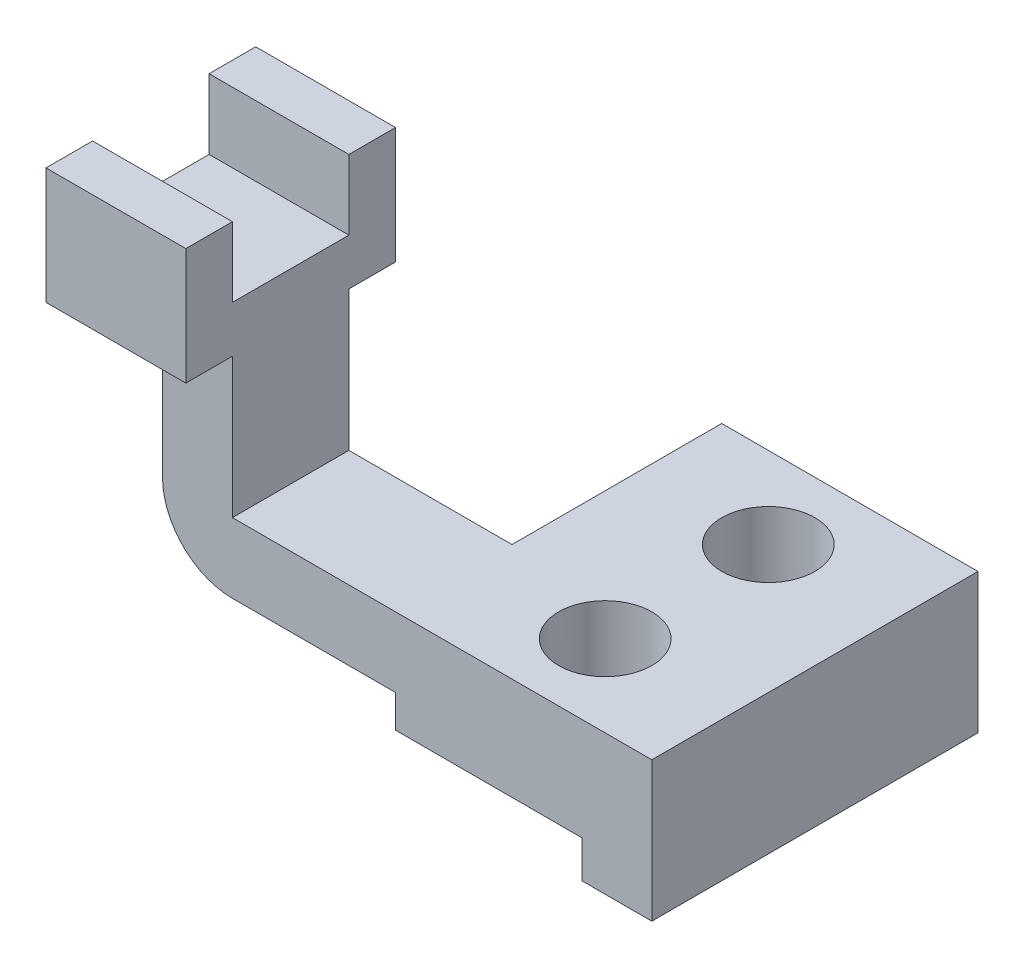
ISO-10303-21;
HEADER;
FILE_DESCRIPTION(('STEP AP214'),'2;1');
FILE_NAME('part.step','',(''),(''),'','','');
FILE_SCHEMA(('AUTOMOTIVE_DESIGN { 1 0 10303 214 1 1 1 1 }'));
ENDSEC;
DATA;
#1=APPLICATION_CONTEXT('core data for automotive mechanical design processes');
#2=APPLICATION_PROTOCOL_DEFINITION('international standard','automotive_design',2000,#1);
#3=PRODUCT_CONTEXT('',#1,'mechanical');
#4=PRODUCT('Part','Part','',(#3));
#5=PRODUCT_RELATED_PRODUCT_CATEGORY('part','',(#4));
#6=PRODUCT_DEFINITION_FORMATION('','',#4);
#7=PRODUCT_DEFINITION_CONTEXT('part definition',#1,'design');
#8=PRODUCT_DEFINITION('design','',#6,#7);
#9=PRODUCT_DEFINITION_SHAPE('','',#8);
#10=(LENGTH_UNIT() NAMED_UNIT(*) SI_UNIT(.MILLI.,.METRE.));
#11=(NAMED_UNIT(*) PLANE_ANGLE_UNIT() SI_UNIT($,.RADIAN.));
#12=(NAMED_UNIT(*) SI_UNIT($,.STERADIAN.) SOLID_ANGLE_UNIT());
#13=UNCERTAINTY_MEASURE_WITH_UNIT(LENGTH_MEASURE(1.E-05),#10,'distance_accuracy_value','');
#14=(GEOMETRIC_REPRESENTATION_CONTEXT(3) GLOBAL_UNCERTAINTY_ASSIGNED_CONTEXT((#13)) GLOBAL_UNIT_ASSIGNED_CONTEXT((#10,
#11,#12)) REPRESENTATION_CONTEXT('',''));
#15=CARTESIAN_POINT('',(0.,0.,0.));
#16=DIRECTION('',(0.,0.,1.));
#17=DIRECTION('',(1.,0.,0.));
#18=AXIS2_PLACEMENT_3D('',#15,#16,#17);
#19=CARTESIAN_POINT('',(-27500.,0.,35000.));
#20=DIRECTION('',(-1.,0.,0.));
#21=DIRECTION('',(0.,0.,1.));
#22=AXIS2_PLACEMENT_3D('',#19,#20,#21);
#23=PLANE('',#22);
#24=DIRECTION('',(0.,1.,0.));
#25=VECTOR('',#24,1.);
#26=CARTESIAN_POINT('',(-27500.,0.,35000.));
#27=LINE('',#26,#25);
#28=CARTESIAN_POINT('',(-27500.,-7000.,35000.));
#29=VERTEX_POINT('',#28);
#30=CARTESIAN_POINT('',(-27500.,-1.77635683940025E-12,35000.));
#31=VERTEX_POINT('',#30);
#32=EDGE_CURVE('E316',#29,#31,#27,.T.);
#33=ORIENTED_EDGE('',*,*,#32,.T.);
#34=DIRECTION('',(0.,0.,-1.));
#35=VECTOR('',#34,1.);
#36=CARTESIAN_POINT('',(-27500.,-1.77635683940025E-12,35000.));
#37=LINE('',#36,#35);
#38=CARTESIAN_POINT('',(-27500.,-1.77635683940025E-12,10000.));
#39=VERTEX_POINT('',#38);
#40=EDGE_CURVE('E282',#31,#39,#37,.T.);
#41=ORIENTED_EDGE('',*,*,#40,.T.);
#42=DIRECTION('',(0.,1.,0.));
#43=VECTOR('',#42,1.);
#44=CARTESIAN_POINT('',(-27500.,-1.77635683940025E-12,10000.));
#45=LINE('',#44,#43);
#46=CARTESIAN_POINT('',(-27500.,15000.,10000.));
#47=VERTEX_POINT('',#46);
#48=EDGE_CURVE('E292',#39,#47,#45,.T.);
#49=ORIENTED_EDGE('',*,*,#48,.T.);
#50=DIRECTION('',(0.,0.,-1.));
#51=VECTOR('',#50,1.);
#52=CARTESIAN_POINT('',(-27500.,15000.,35000.));
#53=LINE('',#52,#51);
#54=CARTESIAN_POINT('',(-27500.,15000.,-35000.));
#55=VERTEX_POINT('',#54);
#56=EDGE_CURVE('E340',#47,#55,#53,.T.);
#57=ORIENTED_EDGE('',*,*,#56,.T.);
#58=DIRECTION('',(0.,1.,0.));
#59=VECTOR('',#58,1.);
#60=CARTESIAN_POINT('',(-27500.,0.,-35000.));
#61=LINE('',#60,#59);
#62=CARTESIAN_POINT('',(-27500.,-7000.,-35000.));
#63=VERTEX_POINT('',#62);
#64=EDGE_CURVE('E304',#63,#55,#61,.T.);
#65=ORIENTED_EDGE('',*,*,#64,.F.);
#66=DIRECTION('',(0.,0.,-1.));
#67=VECTOR('',#66,1.);
#68=CARTESIAN_POINT('',(-27500.,-7000.,35000.));
#69=LINE('',#68,#67);
#70=EDGE_CURVE('E317',#29,#63,#69,.T.);
#71=ORIENTED_EDGE('',*,*,#70,.F.);
#72=EDGE_LOOP('',(#33,#41,#49,#57,#65,#71));
#73=FACE_BOUND('',#72,.T.);
#74=ADVANCED_FACE('F47',(#73),#23,.T.);
#75=CARTESIAN_POINT('',(9.32587340685132E-13,-7000.,35000.));
#76=DIRECTION('',(0.,-1.,0.));
#77=DIRECTION('',(1.,0.,0.));
#78=AXIS2_PLACEMENT_3D('',#75,#76,#77);
#79=PLANE('',#78);
#80=CARTESIAN_POINT('',(0.,-7000.,-17500.));
#81=DIRECTION('',(0.,-1.,0.));
#82=DIRECTION('',(1.,0.,0.));
#83=AXIS2_PLACEMENT_3D('',#80,#81,#82);
#84=CIRCLE('',#83,10000.);
#85=CARTESIAN_POINT('',(10000.,-7000.,-17500.));
#86=VERTEX_POINT('',#85);
#87=EDGE_CURVE('E217',#86,#86,#84,.T.);
#88=ORIENTED_EDGE('',*,*,#87,.F.);
#89=EDGE_LOOP('',(#88));
#90=FACE_BOUND('',#89,.T.);
#91=CARTESIAN_POINT('',(2.14313189850787E-12,-7000.,17500.));
#92=DIRECTION('',(0.,-1.,0.));
#93=DIRECTION('',(1.,0.,0.));
#94=AXIS2_PLACEMENT_3D('',#91,#92,#93);
#95=CIRCLE('',#94,10000.);
#96=CARTESIAN_POINT('',(10000.,-7000.,17500.));
#97=VERTEX_POINT('',#96);
#98=EDGE_CURVE('E743',#97,#97,#95,.T.);
#99=ORIENTED_EDGE('',*,*,#98,.F.);
#100=EDGE_LOOP('',(#99));
#101=FACE_BOUND('',#100,.T.);
#102=DIRECTION('',(-1.,0.,0.));
#103=VECTOR('',#102,1.);
#104=CARTESIAN_POINT('',(9.32587340685132E-13,-7000.,-35000.));
#105=LINE('',#104,#103);
#106=CARTESIAN_POINT('',(12500.,-7000.,-35000.));
#107=VERTEX_POINT('',#106);
#108=EDGE_CURVE('E293',#107,#63,#105,.T.);
#109=ORIENTED_EDGE('',*,*,#108,.F.);
#110=DIRECTION('',(0.,0.,-1.));
#111=VECTOR('',#110,1.);
#112=CARTESIAN_POINT('',(12500.,-7000.,35000.));
#113=LINE('',#112,#111);
#114=CARTESIAN_POINT('',(12500.,-7000.,35000.));
#115=VERTEX_POINT('',#114);
#116=EDGE_CURVE('E344',#115,#107,#113,.T.);
#117=ORIENTED_EDGE('',*,*,#116,.F.);
#118=DIRECTION('',(-1.,0.,0.));
#119=VECTOR('',#118,1.);
#120=CARTESIAN_POINT('',(9.32587340685132E-13,-7000.,35000.));
#121=LINE('',#120,#119);
#122=EDGE_CURVE('E301',#115,#29,#121,.T.);
#123=ORIENTED_EDGE('',*,*,#122,.T.);
#124=ORIENTED_EDGE('',*,*,#70,.T.);
#125=EDGE_LOOP('',(#109,#117,#123,#124));
#126=FACE_BOUND('',#125,.T.);
#127=ADVANCED_FACE('F380',(#90,#101,#126),#79,.T.);
#128=CARTESIAN_POINT('',(12500.,0.,35000.));
#129=DIRECTION('',(-1.,0.,0.));
#130=DIRECTION('',(0.,0.,1.));
#131=AXIS2_PLACEMENT_3D('',#128,#129,#130);
#132=PLANE('',#131);
#133=DIRECTION('',(0.,1.,0.));
#134=VECTOR('',#133,1.);
#135=CARTESIAN_POINT('',(12500.,0.,-35000.));
#136=LINE('',#135,#134);
#137=CARTESIAN_POINT('',(12500.,-15000.,-35000.));
#138=VERTEX_POINT('',#137);
#139=EDGE_CURVE('E325',#138,#107,#136,.T.);
#140=ORIENTED_EDGE('',*,*,#139,.F.);
#141=DIRECTION('',(0.,0.,-1.));
#142=VECTOR('',#141,1.);
#143=CARTESIAN_POINT('',(12500.,-15000.,35000.));
#144=LINE('',#143,#142);
#145=CARTESIAN_POINT('',(12500.,-15000.,35000.));
#146=VERTEX_POINT('',#145);
#147=EDGE_CURVE('E343',#146,#138,#144,.T.);
#148=ORIENTED_EDGE('',*,*,#147,.F.);
#149=DIRECTION('',(0.,1.,0.));
#150=VECTOR('',#149,1.);
#151=CARTESIAN_POINT('',(12500.,0.,35000.));
#152=LINE('',#151,#150);
#153=EDGE_CURVE('E302',#146,#115,#152,.T.);
#154=ORIENTED_EDGE('',*,*,#153,.T.);
#155=ORIENTED_EDGE('',*,*,#116,.T.);
#156=EDGE_LOOP('',(#140,#148,#154,#155));
#157=FACE_BOUND('',#156,.T.);
#158=ADVANCED_FACE('F382',(#157),#132,.T.);
#159=CARTESIAN_POINT('',(0.,-15000.,35000.));
#160=DIRECTION('',(0.,-1.,0.));
#161=DIRECTION('',(0.,0.,-1.));
#162=AXIS2_PLACEMENT_3D('',#159,#160,#161);
#163=PLANE('',#162);
#164=DIRECTION('',(-1.,0.,0.));
#165=VECTOR('',#164,1.);
#166=CARTESIAN_POINT('',(0.,-15000.,-35000.));
#167=LINE('',#166,#165);
#168=CARTESIAN_POINT('',(27500.,-15000.,-35000.));
#169=VERTEX_POINT('',#168);
#170=EDGE_CURVE('E324',#169,#138,#167,.T.);
#171=ORIENTED_EDGE('',*,*,#170,.F.);
#172=DIRECTION('',(0.,0.,-1.));
#173=VECTOR('',#172,1.);
#174=CARTESIAN_POINT('',(27500.,-15000.,35000.));
#175=LINE('',#174,#173);
#176=CARTESIAN_POINT('',(27500.,-15000.,35000.));
#177=VERTEX_POINT('',#176);
#178=EDGE_CURVE('E341',#177,#169,#175,.T.);
#179=ORIENTED_EDGE('',*,*,#178,.F.);
#180=DIRECTION('',(-1.,0.,0.));
#181=VECTOR('',#180,1.);
#182=CARTESIAN_POINT('',(0.,-15000.,35000.));
#183=LINE('',#182,#181);
#184=EDGE_CURVE('E306',#177,#146,#183,.T.);
#185=ORIENTED_EDGE('',*,*,#184,.T.);
#186=ORIENTED_EDGE('',*,*,#147,.T.);
#187=EDGE_LOOP('',(#171,#179,#185,#186));
#188=FACE_BOUND('',#187,.T.);
#189=ADVANCED_FACE('F396',(#188),#163,.T.);
#190=CARTESIAN_POINT('',(27500.,6.51330841113425E-12,35000.));
#191=DIRECTION('',(1.,0.,0.));
#192=DIRECTION('',(0.,1.,0.));
#193=AXIS2_PLACEMENT_3D('',#190,#191,#192);
#194=PLANE('',#193);
#195=DIRECTION('',(0.,-1.,0.));
#196=VECTOR('',#195,1.);
#197=CARTESIAN_POINT('',(27500.,6.51330841113425E-12,-35000.));
#198=LINE('',#197,#196);
#199=CARTESIAN_POINT('',(27500.,15000.,-35000.));
#200=VERTEX_POINT('',#199);
#201=EDGE_CURVE('E327',#200,#169,#198,.T.);
#202=ORIENTED_EDGE('',*,*,#201,.F.);
#203=DIRECTION('',(0.,0.,-1.));
#204=VECTOR('',#203,1.);
#205=CARTESIAN_POINT('',(27500.,15000.,35000.));
#206=LINE('',#205,#204);
#207=CARTESIAN_POINT('',(27500.,15000.,35000.));
#208=VERTEX_POINT('',#207);
#209=EDGE_CURVE('E337',#208,#200,#206,.T.);
#210=ORIENTED_EDGE('',*,*,#209,.F.);
#211=DIRECTION('',(0.,-1.,0.));
#212=VECTOR('',#211,1.);
#213=CARTESIAN_POINT('',(27500.,6.51330841113425E-12,35000.));
#214=LINE('',#213,#212);
#215=EDGE_CURVE('E313',#208,#177,#214,.T.);
#216=ORIENTED_EDGE('',*,*,#215,.T.);
#217=ORIENTED_EDGE('',*,*,#178,.T.);
#218=EDGE_LOOP('',(#202,#210,#216,#217));
#219=FACE_BOUND('',#218,.T.);
#220=ADVANCED_FACE('F395',(#219),#194,.T.);
#221=CARTESIAN_POINT('',(0.,15000.,35000.));
#222=DIRECTION('',(0.,1.,0.));
#223=DIRECTION('',(0.,0.,1.));
#224=AXIS2_PLACEMENT_3D('',#221,#222,#223);
#225=PLANE('',#224);
#226=CARTESIAN_POINT('',(0.,15000.,-17500.));
#227=DIRECTION('',(0.,1.,0.));
#228=DIRECTION('',(0.,0.,1.));
#229=AXIS2_PLACEMENT_3D('',#226,#227,#228);
#230=CIRCLE('',#229,10000.);
#231=CARTESIAN_POINT('',(0.,15000.,-7500.));
#232=VERTEX_POINT('',#231);
#233=EDGE_CURVE('E745',#232,#232,#230,.T.);
#234=ORIENTED_EDGE('',*,*,#233,.F.);
#235=EDGE_LOOP('',(#234));
#236=FACE_BOUND('',#235,.T.);
#237=CARTESIAN_POINT('',(2.14313189850787E-12,15000.,17500.));
#238=DIRECTION('',(0.,1.,0.));
#239=DIRECTION('',(0.,0.,1.));
#240=AXIS2_PLACEMENT_3D('',#237,#238,#239);
#241=CIRCLE('',#240,10000.);
#242=CARTESIAN_POINT('',(2.14313189850787E-12,15000.,27500.));
#243=VERTEX_POINT('',#242);
#244=EDGE_CURVE('E742',#243,#243,#241,.T.);
#245=ORIENTED_EDGE('',*,*,#244,.F.);
#246=EDGE_LOOP('',(#245));
#247=FACE_BOUND('',#246,.T.);
#248=DIRECTION('',(0.,0.,-1.));
#249=VECTOR('',#248,1.);
#250=CARTESIAN_POINT('',(-62500.,15000.,35000.));
#251=LINE('',#250,#249);
#252=CARTESIAN_POINT('',(-62500.,15000.,35000.));
#253=VERTEX_POINT('',#252);
#254=CARTESIAN_POINT('',(-62500.,15000.,10000.));
#255=VERTEX_POINT('',#254);
#256=EDGE_CURVE('E255',#253,#255,#251,.T.);
#257=ORIENTED_EDGE('',*,*,#256,.F.);
#258=DIRECTION('',(1.,0.,0.));
#259=VECTOR('',#258,1.);
#260=CARTESIAN_POINT('',(0.,15000.,35000.));
#261=LINE('',#260,#259);
#262=EDGE_CURVE('E314',#253,#208,#261,.T.);
#263=ORIENTED_EDGE('',*,*,#262,.T.);
#264=ORIENTED_EDGE('',*,*,#209,.T.);
#265=DIRECTION('',(1.,0.,0.));
#266=VECTOR('',#265,1.);
#267=CARTESIAN_POINT('',(0.,15000.,-35000.));
#268=LINE('',#267,#266);
#269=EDGE_CURVE('E332',#55,#200,#268,.T.);
#270=ORIENTED_EDGE('',*,*,#269,.F.);
#271=ORIENTED_EDGE('',*,*,#56,.F.);
#272=DIRECTION('',(-1.,0.,0.));
#273=VECTOR('',#272,1.);
#274=CARTESIAN_POINT('',(-27500.,15000.,10000.));
#275=LINE('',#274,#273);
#276=EDGE_CURVE('E281',#47,#255,#275,.T.);
#277=ORIENTED_EDGE('',*,*,#276,.T.);
#278=EDGE_LOOP('',(#257,#263,#264,#270,#271,#277));
#279=FACE_BOUND('',#278,.T.);
#280=ADVANCED_FACE('F386',(#236,#247,#279),#225,.T.);
#281=CARTESIAN_POINT('',(0.,0.,35000.));
#282=DIRECTION('',(0.,0.,1.));
#283=DIRECTION('',(1.,0.,0.));
#284=AXIS2_PLACEMENT_3D('',#281,#282,#283);
#285=PLANE('',#284);
#286=DIRECTION('',(0.,1.,0.));
#287=VECTOR('',#286,1.);
#288=CARTESIAN_POINT('',(-77500.,-1.77635683940025E-12,35000.));
#289=LINE('',#288,#287);
#290=CARTESIAN_POINT('',(-77500.,15000.,35000.));
#291=VERTEX_POINT('',#290);
#292=CARTESIAN_POINT('',(-77500.,45000.,35000.));
#293=VERTEX_POINT('',#292);
#294=EDGE_CURVE('E291',#291,#293,#289,.T.);
#295=ORIENTED_EDGE('',*,*,#294,.F.);
#296=CARTESIAN_POINT('',(-62500.,15000.,35000.));
#297=DIRECTION('',(0.,0.,1.));
#298=DIRECTION('',(1.,0.,0.));
#299=AXIS2_PLACEMENT_3D('',#296,#297,#298);
#300=CIRCLE('',#299,15000.);
#301=CARTESIAN_POINT('',(-62500.,-1.77635683940025E-12,35000.));
#302=VERTEX_POINT('',#301);
#303=EDGE_CURVE('E72',#291,#302,#300,.T.);
#304=ORIENTED_EDGE('',*,*,#303,.T.);
#305=DIRECTION('',(1.,0.,0.));
#306=VECTOR('',#305,1.);
#307=CARTESIAN_POINT('',(-27500.,-1.77635683940025E-12,35000.));
#308=LINE('',#307,#306);
#309=EDGE_CURVE('E287',#302,#31,#308,.T.);
#310=ORIENTED_EDGE('',*,*,#309,.T.);
#311=ORIENTED_EDGE('',*,*,#32,.F.);
#312=ORIENTED_EDGE('',*,*,#122,.F.);
#313=ORIENTED_EDGE('',*,*,#153,.F.);
#314=ORIENTED_EDGE('',*,*,#184,.F.);
#315=ORIENTED_EDGE('',*,*,#215,.F.);
#316=ORIENTED_EDGE('',*,*,#262,.F.);
#317=DIRECTION('',(0.,-1.,0.));
#318=VECTOR('',#317,1.);
#319=CARTESIAN_POINT('',(-62500.,45000.,35000.));
#320=LINE('',#319,#318);
#321=CARTESIAN_POINT('',(-62500.,45000.,35000.));
#322=VERTEX_POINT('',#321);
#323=EDGE_CURVE('E278',#322,#253,#320,.T.);
#324=ORIENTED_EDGE('',*,*,#323,.F.);
#325=DIRECTION('',(1.,0.,0.));
#326=VECTOR('',#325,1.);
#327=CARTESIAN_POINT('',(-77500.,45000.,35000.));
#328=LINE('',#327,#326);
#329=EDGE_CURVE('E267',#293,#322,#328,.T.);
#330=ORIENTED_EDGE('',*,*,#329,.F.);
#331=EDGE_LOOP('',(#295,#304,#310,#311,#312,#313,#314,#315,#316,#324,#330));
#332=FACE_BOUND('',#331,.T.);
#333=ADVANCED_FACE('F360',(#332),#285,.T.);
#334=CARTESIAN_POINT('',(0.,0.,-35000.));
#335=DIRECTION('',(0.,0.,1.));
#336=DIRECTION('',(1.,0.,0.));
#337=AXIS2_PLACEMENT_3D('',#334,#335,#336);
#338=PLANE('',#337);
#339=ORIENTED_EDGE('',*,*,#108,.T.);
#340=ORIENTED_EDGE('',*,*,#64,.T.);
#341=ORIENTED_EDGE('',*,*,#269,.T.);
#342=ORIENTED_EDGE('',*,*,#201,.T.);
#343=ORIENTED_EDGE('',*,*,#170,.T.);
#344=ORIENTED_EDGE('',*,*,#139,.T.);
#345=EDGE_LOOP('',(#339,#340,#341,#342,#343,#344));
#346=FACE_BOUND('',#345,.T.);
#347=ADVANCED_FACE('F390',(#346),#338,.F.);
#348=CARTESIAN_POINT('',(-77500.,-1.77635683940025E-12,35000.));
#349=DIRECTION('',(-1.,0.,0.));
#350=DIRECTION('',(0.,0.,1.));
#351=AXIS2_PLACEMENT_3D('',#348,#349,#350);
#352=PLANE('',#351);
#353=DIRECTION('',(0.,1.,0.));
#354=VECTOR('',#353,1.);
#355=CARTESIAN_POINT('',(-77500.,-1.77635683940025E-12,10000.));
#356=LINE('',#355,#354);
#357=CARTESIAN_POINT('',(-77500.,15000.,10000.));
#358=VERTEX_POINT('',#357);
#359=CARTESIAN_POINT('',(-77500.,45000.,10000.));
#360=VERTEX_POINT('',#359);
#361=EDGE_CURVE('E298',#358,#360,#356,.T.);
#362=ORIENTED_EDGE('',*,*,#361,.F.);
#363=DIRECTION('',(0.,0.,1.));
#364=VECTOR('',#363,1.);
#365=CARTESIAN_POINT('',(-77500.,15000.,35000.));
#366=LINE('',#365,#364);
#367=EDGE_CURVE('E350',#358,#291,#366,.T.);
#368=ORIENTED_EDGE('',*,*,#367,.T.);
#369=ORIENTED_EDGE('',*,*,#294,.T.);
#370=DIRECTION('',(0.,0.,1.));
#371=VECTOR('',#370,1.);
#372=CARTESIAN_POINT('',(-77500.,45000.,35000.));
#373=LINE('',#372,#371);
#374=EDGE_CURVE('E266',#360,#293,#373,.T.);
#375=ORIENTED_EDGE('',*,*,#374,.F.);
#376=EDGE_LOOP('',(#362,#368,#369,#375));
#377=FACE_BOUND('',#376,.T.);
#378=ADVANCED_FACE('F351',(#377),#352,.T.);
#379=CARTESIAN_POINT('',(-27500.,-1.77635683940025E-12,10000.));
#380=DIRECTION('',(0.,0.,-1.));
#381=DIRECTION('',(-1.,0.,0.));
#382=AXIS2_PLACEMENT_3D('',#379,#380,#381);
#383=PLANE('',#382);
#384=DIRECTION('',(-1.,0.,0.));
#385=VECTOR('',#384,1.);
#386=CARTESIAN_POINT('',(-27500.,-1.77635683940025E-12,10000.));
#387=LINE('',#386,#385);
#388=CARTESIAN_POINT('',(-62500.,-1.77635683940025E-12,10000.));
#389=VERTEX_POINT('',#388);
#390=EDGE_CURVE('E290',#39,#389,#387,.T.);
#391=ORIENTED_EDGE('',*,*,#390,.T.);
#392=CARTESIAN_POINT('',(-62500.,15000.,10000.));
#393=DIRECTION('',(0.,0.,-1.));
#394=DIRECTION('',(-1.,0.,0.));
#395=AXIS2_PLACEMENT_3D('',#392,#393,#394);
#396=CIRCLE('',#395,15000.);
#397=EDGE_CURVE('E11',#389,#358,#396,.T.);
#398=ORIENTED_EDGE('',*,*,#397,.T.);
#399=ORIENTED_EDGE('',*,*,#361,.T.);
#400=DIRECTION('',(-1.,0.,0.));
#401=VECTOR('',#400,1.);
#402=CARTESIAN_POINT('',(-77500.,45000.,10000.));
#403=LINE('',#402,#401);
#404=CARTESIAN_POINT('',(-62500.,45000.,10000.));
#405=VERTEX_POINT('',#404);
#406=EDGE_CURVE('E275',#405,#360,#403,.T.);
#407=ORIENTED_EDGE('',*,*,#406,.F.);
#408=DIRECTION('',(0.,-1.,0.));
#409=VECTOR('',#408,1.);
#410=CARTESIAN_POINT('',(-62500.,45000.,10000.));
#411=LINE('',#410,#409);
#412=EDGE_CURVE('E274',#405,#255,#411,.T.);
#413=ORIENTED_EDGE('',*,*,#412,.T.);
#414=ORIENTED_EDGE('',*,*,#276,.F.);
#415=ORIENTED_EDGE('',*,*,#48,.F.);
#416=EDGE_LOOP('',(#391,#398,#399,#407,#413,#414,#415));
#417=FACE_BOUND('',#416,.T.);
#418=ADVANCED_FACE('F364',(#417),#383,.T.);
#419=CARTESIAN_POINT('',(0.,-1.77635683940025E-12,0.));
#420=DIRECTION('',(0.,1.,0.));
#421=DIRECTION('',(0.,0.,1.));
#422=AXIS2_PLACEMENT_3D('',#419,#420,#421);
#423=PLANE('',#422);
#424=ORIENTED_EDGE('',*,*,#309,.F.);
#425=DIRECTION('',(0.,0.,1.));
#426=VECTOR('',#425,1.);
#427=CARTESIAN_POINT('',(-62500.,-1.77635683940025E-12,10000.));
#428=LINE('',#427,#426);
#429=EDGE_CURVE('E60',#302,#389,#428,.F.);
#430=ORIENTED_EDGE('',*,*,#429,.T.);
#431=ORIENTED_EDGE('',*,*,#390,.F.);
#432=ORIENTED_EDGE('',*,*,#40,.F.);
#433=EDGE_LOOP('',(#424,#430,#431,#432));
#434=FACE_BOUND('',#433,.T.);
#435=ADVANCED_FACE('F373',(#434),#423,.F.);
#436=CARTESIAN_POINT('',(-62500.,45000.,35000.));
#437=DIRECTION('',(-1.,0.,0.));
#438=DIRECTION('',(0.,0.,1.));
#439=AXIS2_PLACEMENT_3D('',#436,#437,#438);
#440=PLANE('',#439);
#441=ORIENTED_EDGE('',*,*,#256,.T.);
#442=ORIENTED_EDGE('',*,*,#412,.F.);
#443=DIRECTION('',(0.,0.,-1.));
#444=VECTOR('',#443,1.);
#445=CARTESIAN_POINT('',(-62500.,45000.,1.4210854715202E-11));
#446=LINE('',#445,#444);
#447=CARTESIAN_POINT('',(-62500.,45000.,1.4210854715202E-11));
#448=VERTEX_POINT('',#447);
#449=EDGE_CURVE('E214',#405,#448,#446,.T.);
#450=ORIENTED_EDGE('',*,*,#449,.T.);
#451=DIRECTION('',(0.,1.,0.));
#452=VECTOR('',#451,1.);
#453=CARTESIAN_POINT('',(-62500.,45000.,1.4210854715202E-11));
#454=LINE('',#453,#452);
#455=CARTESIAN_POINT('',(-62500.,70000.,1.4210854715202E-11));
#456=VERTEX_POINT('',#455);
#457=EDGE_CURVE('E234',#448,#456,#454,.T.);
#458=ORIENTED_EDGE('',*,*,#457,.T.);
#459=DIRECTION('',(0.,0.,1.));
#460=VECTOR('',#459,1.);
#461=CARTESIAN_POINT('',(-62500.,70000.,1.4210854715202E-11));
#462=LINE('',#461,#460);
#463=CARTESIAN_POINT('',(-62500.,70000.,10000.));
#464=VERTEX_POINT('',#463);
#465=EDGE_CURVE('E189',#456,#464,#462,.T.);
#466=ORIENTED_EDGE('',*,*,#465,.T.);
#467=DIRECTION('',(0.,-1.,0.));
#468=VECTOR('',#467,1.);
#469=CARTESIAN_POINT('',(-62500.,70000.,10000.));
#470=LINE('',#469,#468);
#471=CARTESIAN_POINT('',(-62500.,55000.,10000.));
#472=VERTEX_POINT('',#471);
#473=EDGE_CURVE('E236',#464,#472,#470,.T.);
#474=ORIENTED_EDGE('',*,*,#473,.T.);
#475=DIRECTION('',(0.,0.,1.));
#476=VECTOR('',#475,1.);
#477=CARTESIAN_POINT('',(-62500.,55000.,10000.));
#478=LINE('',#477,#476);
#479=CARTESIAN_POINT('',(-62500.,55000.,35000.));
#480=VERTEX_POINT('',#479);
#481=EDGE_CURVE('E243',#472,#480,#478,.T.);
#482=ORIENTED_EDGE('',*,*,#481,.T.);
#483=DIRECTION('',(0.,1.,0.));
#484=VECTOR('',#483,1.);
#485=CARTESIAN_POINT('',(-62500.,55000.,35000.));
#486=LINE('',#485,#484);
#487=CARTESIAN_POINT('',(-62500.,70000.,35000.));
#488=VERTEX_POINT('',#487);
#489=EDGE_CURVE('E242',#480,#488,#486,.T.);
#490=ORIENTED_EDGE('',*,*,#489,.T.);
#491=DIRECTION('',(0.,0.,1.));
#492=VECTOR('',#491,1.);
#493=CARTESIAN_POINT('',(-62500.,70000.,35000.));
#494=LINE('',#493,#492);
#495=CARTESIAN_POINT('',(-62500.,70000.,45000.));
#496=VERTEX_POINT('',#495);
#497=EDGE_CURVE('E250',#488,#496,#494,.T.);
#498=ORIENTED_EDGE('',*,*,#497,.T.);
#499=DIRECTION('',(0.,-1.,0.));
#500=VECTOR('',#499,1.);
#501=CARTESIAN_POINT('',(-62500.,45000.,45000.));
#502=LINE('',#501,#500);
#503=CARTESIAN_POINT('',(-62500.,45000.,45000.));
#504=VERTEX_POINT('',#503);
#505=EDGE_CURVE('E249',#496,#504,#502,.T.);
#506=ORIENTED_EDGE('',*,*,#505,.T.);
#507=EDGE_CURVE('E215',#504,#322,#446,.T.);
#508=ORIENTED_EDGE('',*,*,#507,.T.);
#509=ORIENTED_EDGE('',*,*,#323,.T.);
#510=EDGE_LOOP('',(#441,#442,#450,#458,#466,#474,#482,#490,#498,#506,#508,#509));
#511=FACE_BOUND('',#510,.T.);
#512=ADVANCED_FACE('F370',(#511),#440,.F.);
#513=CARTESIAN_POINT('',(-62500.,15000.,35000.));
#514=DIRECTION('',(0.,0.,-1.));
#515=DIRECTION('',(-1.,0.,0.));
#516=AXIS2_PLACEMENT_3D('',#513,#514,#515);
#517=CYLINDRICAL_SURFACE('',#516,15000.);
#518=ORIENTED_EDGE('',*,*,#397,.F.);
#519=ORIENTED_EDGE('',*,*,#429,.F.);
#520=ORIENTED_EDGE('',*,*,#303,.F.);
#521=ORIENTED_EDGE('',*,*,#367,.F.);
#522=EDGE_LOOP('',(#518,#519,#520,#521));
#523=FACE_BOUND('',#522,.T.);
#524=ADVANCED_FACE('F51',(#523),#517,.T.);
#525=CARTESIAN_POINT('',(-92500.,45000.,1.4210854715202E-11));
#526=DIRECTION('',(0.,0.,-1.));
#527=DIRECTION('',(-1.,0.,0.));
#528=AXIS2_PLACEMENT_3D('',#525,#526,#527);
#529=PLANE('',#528);
#530=ORIENTED_EDGE('',*,*,#457,.F.);
#531=DIRECTION('',(1.,0.,0.));
#532=VECTOR('',#531,1.);
#533=CARTESIAN_POINT('',(-92500.,45000.,1.4210854715202E-11));
#534=LINE('',#533,#532);
#535=CARTESIAN_POINT('',(-92500.,45000.,1.4210854715202E-11));
#536=VERTEX_POINT('',#535);
#537=EDGE_CURVE('E211',#536,#448,#534,.T.);
#538=ORIENTED_EDGE('',*,*,#537,.F.);
#539=DIRECTION('',(0.,1.,0.));
#540=VECTOR('',#539,1.);
#541=CARTESIAN_POINT('',(-92500.,45000.,1.4210854715202E-11));
#542=LINE('',#541,#540);
#543=CARTESIAN_POINT('',(-92500.,70000.,1.4210854715202E-11));
#544=VERTEX_POINT('',#543);
#545=EDGE_CURVE('E201',#536,#544,#542,.T.);
#546=ORIENTED_EDGE('',*,*,#545,.T.);
#547=DIRECTION('',(1.,0.,0.));
#548=VECTOR('',#547,1.);
#549=CARTESIAN_POINT('',(-92500.,70000.,1.4210854715202E-11));
#550=LINE('',#549,#548);
#551=EDGE_CURVE('E183',#544,#456,#550,.T.);
#552=ORIENTED_EDGE('',*,*,#551,.T.);
#553=EDGE_LOOP('',(#530,#538,#546,#552));
#554=FACE_BOUND('',#553,.T.);
#555=ADVANCED_FACE('F207',(#554),#529,.T.);
#556=CARTESIAN_POINT('',(-92500.,45000.,1.4210854715202E-11));
#557=DIRECTION('',(0.,-1.,0.));
#558=DIRECTION('',(0.,0.,-1.));
#559=AXIS2_PLACEMENT_3D('',#556,#557,#558);
#560=PLANE('',#559);
#561=ORIENTED_EDGE('',*,*,#374,.T.);
#562=ORIENTED_EDGE('',*,*,#329,.T.);
#563=ORIENTED_EDGE('',*,*,#507,.F.);
#564=DIRECTION('',(1.,0.,0.));
#565=VECTOR('',#564,1.);
#566=CARTESIAN_POINT('',(-92500.,45000.,45000.));
#567=LINE('',#566,#565);
#568=CARTESIAN_POINT('',(-92500.,45000.,45000.));
#569=VERTEX_POINT('',#568);
#570=EDGE_CURVE('E254',#569,#504,#567,.T.);
#571=ORIENTED_EDGE('',*,*,#570,.F.);
#572=DIRECTION('',(0.,0.,-1.));
#573=VECTOR('',#572,1.);
#574=CARTESIAN_POINT('',(-92500.,45000.,1.4210854715202E-11));
#575=LINE('',#574,#573);
#576=EDGE_CURVE('E198',#569,#536,#575,.T.);
#577=ORIENTED_EDGE('',*,*,#576,.T.);
#578=ORIENTED_EDGE('',*,*,#537,.T.);
#579=ORIENTED_EDGE('',*,*,#449,.F.);
#580=ORIENTED_EDGE('',*,*,#406,.T.);
#581=EDGE_LOOP('',(#561,#562,#563,#571,#577,#578,#579,#580));
#582=FACE_BOUND('',#581,.T.);
#583=ADVANCED_FACE('F363',(#582),#560,.T.);
#584=CARTESIAN_POINT('',(-92500.,45000.,45000.));
#585=DIRECTION('',(0.,0.,1.));
#586=DIRECTION('',(1.,0.,0.));
#587=AXIS2_PLACEMENT_3D('',#584,#585,#586);
#588=PLANE('',#587);
#589=ORIENTED_EDGE('',*,*,#505,.F.);
#590=DIRECTION('',(1.,0.,0.));
#591=VECTOR('',#590,1.);
#592=CARTESIAN_POINT('',(-92500.,70000.,45000.));
#593=LINE('',#592,#591);
#594=CARTESIAN_POINT('',(-92500.,70000.,45000.));
#595=VERTEX_POINT('',#594);
#596=EDGE_CURVE('E260',#595,#496,#593,.T.);
#597=ORIENTED_EDGE('',*,*,#596,.F.);
#598=DIRECTION('',(0.,-1.,0.));
#599=VECTOR('',#598,1.);
#600=CARTESIAN_POINT('',(-92500.,45000.,45000.));
#601=LINE('',#600,#599);
#602=EDGE_CURVE('E231',#595,#569,#601,.T.);
#603=ORIENTED_EDGE('',*,*,#602,.T.);
#604=ORIENTED_EDGE('',*,*,#570,.T.);
#605=EDGE_LOOP('',(#589,#597,#603,#604));
#606=FACE_BOUND('',#605,.T.);
#607=ADVANCED_FACE('F423',(#606),#588,.T.);
#608=CARTESIAN_POINT('',(-92500.,70000.,35000.));
#609=DIRECTION('',(0.,1.,0.));
#610=DIRECTION('',(0.,0.,1.));
#611=AXIS2_PLACEMENT_3D('',#608,#609,#610);
#612=PLANE('',#611);
#613=ORIENTED_EDGE('',*,*,#497,.F.);
#614=DIRECTION('',(1.,0.,0.));
#615=VECTOR('',#614,1.);
#616=CARTESIAN_POINT('',(-92500.,70000.,35000.));
#617=LINE('',#616,#615);
#618=CARTESIAN_POINT('',(-92500.,70000.,35000.));
#619=VERTEX_POINT('',#618);
#620=EDGE_CURVE('E259',#619,#488,#617,.T.);
#621=ORIENTED_EDGE('',*,*,#620,.F.);
#622=DIRECTION('',(0.,0.,1.));
#623=VECTOR('',#622,1.);
#624=CARTESIAN_POINT('',(-92500.,70000.,35000.));
#625=LINE('',#624,#623);
#626=EDGE_CURVE('E226',#619,#595,#625,.T.);
#627=ORIENTED_EDGE('',*,*,#626,.T.);
#628=ORIENTED_EDGE('',*,*,#596,.T.);
#629=EDGE_LOOP('',(#613,#621,#627,#628));
#630=FACE_BOUND('',#629,.T.);
#631=ADVANCED_FACE('F426',(#630),#612,.T.);
#632=CARTESIAN_POINT('',(-92500.,55000.,35000.));
#633=DIRECTION('',(0.,0.,-1.));
#634=DIRECTION('',(-1.,0.,0.));
#635=AXIS2_PLACEMENT_3D('',#632,#633,#634);
#636=PLANE('',#635);
#637=ORIENTED_EDGE('',*,*,#489,.F.);
#638=DIRECTION('',(1.,0.,0.));
#639=VECTOR('',#638,1.);
#640=CARTESIAN_POINT('',(-92500.,55000.,35000.));
#641=LINE('',#640,#639);
#642=CARTESIAN_POINT('',(-92500.,55000.,35000.));
#643=VERTEX_POINT('',#642);
#644=EDGE_CURVE('E261',#643,#480,#641,.T.);
#645=ORIENTED_EDGE('',*,*,#644,.F.);
#646=DIRECTION('',(0.,1.,0.));
#647=VECTOR('',#646,1.);
#648=CARTESIAN_POINT('',(-92500.,55000.,35000.));
#649=LINE('',#648,#647);
#650=EDGE_CURVE('E223',#643,#619,#649,.T.);
#651=ORIENTED_EDGE('',*,*,#650,.T.);
#652=ORIENTED_EDGE('',*,*,#620,.T.);
#653=EDGE_LOOP('',(#637,#645,#651,#652));
#654=FACE_BOUND('',#653,.T.);
#655=ADVANCED_FACE('F427',(#654),#636,.T.);
#656=CARTESIAN_POINT('',(-92500.,55000.,10000.));
#657=DIRECTION('',(0.,1.,0.));
#658=DIRECTION('',(0.,0.,1.));
#659=AXIS2_PLACEMENT_3D('',#656,#657,#658);
#660=PLANE('',#659);
#661=ORIENTED_EDGE('',*,*,#481,.F.);
#662=DIRECTION('',(1.,0.,0.));
#663=VECTOR('',#662,1.);
#664=CARTESIAN_POINT('',(-92500.,55000.,10000.));
#665=LINE('',#664,#663);
#666=CARTESIAN_POINT('',(-92500.,55000.,10000.));
#667=VERTEX_POINT('',#666);
#668=EDGE_CURVE('E263',#667,#472,#665,.T.);
#669=ORIENTED_EDGE('',*,*,#668,.F.);
#670=DIRECTION('',(0.,0.,1.));
#671=VECTOR('',#670,1.);
#672=CARTESIAN_POINT('',(-92500.,55000.,10000.));
#673=LINE('',#672,#671);
#674=EDGE_CURVE('E225',#667,#643,#673,.T.);
#675=ORIENTED_EDGE('',*,*,#674,.T.);
#676=ORIENTED_EDGE('',*,*,#644,.T.);
#677=EDGE_LOOP('',(#661,#669,#675,#676));
#678=FACE_BOUND('',#677,.T.);
#679=ADVANCED_FACE('F435',(#678),#660,.T.);
#680=CARTESIAN_POINT('',(-92500.,70000.,10000.));
#681=DIRECTION('',(0.,0.,1.));
#682=DIRECTION('',(0.,-1.,0.));
#683=AXIS2_PLACEMENT_3D('',#680,#681,#682);
#684=PLANE('',#683);
#685=ORIENTED_EDGE('',*,*,#473,.F.);
#686=DIRECTION('',(1.,0.,0.));
#687=VECTOR('',#686,1.);
#688=CARTESIAN_POINT('',(-92500.,70000.,10000.));
#689=LINE('',#688,#687);
#690=CARTESIAN_POINT('',(-92500.,70000.,10000.));
#691=VERTEX_POINT('',#690);
#692=EDGE_CURVE('E194',#691,#464,#689,.T.);
#693=ORIENTED_EDGE('',*,*,#692,.F.);
#694=DIRECTION('',(0.,-1.,0.));
#695=VECTOR('',#694,1.);
#696=CARTESIAN_POINT('',(-92500.,70000.,10000.));
#697=LINE('',#696,#695);
#698=EDGE_CURVE('E210',#691,#667,#697,.T.);
#699=ORIENTED_EDGE('',*,*,#698,.T.);
#700=ORIENTED_EDGE('',*,*,#668,.T.);
#701=EDGE_LOOP('',(#685,#693,#699,#700));
#702=FACE_BOUND('',#701,.T.);
#703=ADVANCED_FACE('F434',(#702),#684,.T.);
#704=CARTESIAN_POINT('',(-92500.,70000.,1.4210854715202E-11));
#705=DIRECTION('',(0.,1.,0.));
#706=DIRECTION('',(0.,0.,1.));
#707=AXIS2_PLACEMENT_3D('',#704,#705,#706);
#708=PLANE('',#707);
#709=ORIENTED_EDGE('',*,*,#465,.F.);
#710=ORIENTED_EDGE('',*,*,#551,.F.);
#711=DIRECTION('',(0.,0.,1.));
#712=VECTOR('',#711,1.);
#713=CARTESIAN_POINT('',(-92500.,70000.,1.4210854715202E-11));
#714=LINE('',#713,#712);
#715=EDGE_CURVE('E186',#544,#691,#714,.T.);
#716=ORIENTED_EDGE('',*,*,#715,.T.);
#717=ORIENTED_EDGE('',*,*,#692,.T.);
#718=EDGE_LOOP('',(#709,#710,#716,#717));
#719=FACE_BOUND('',#718,.T.);
#720=ADVANCED_FACE('F190',(#719),#708,.T.);
#721=CARTESIAN_POINT('',(-92500.,0.,0.));
#722=DIRECTION('',(1.,0.,0.));
#723=DIRECTION('',(0.,0.,-1.));
#724=AXIS2_PLACEMENT_3D('',#721,#722,#723);
#725=PLANE('',#724);
#726=ORIENTED_EDGE('',*,*,#545,.F.);
#727=ORIENTED_EDGE('',*,*,#576,.F.);
#728=ORIENTED_EDGE('',*,*,#602,.F.);
#729=ORIENTED_EDGE('',*,*,#626,.F.);
#730=ORIENTED_EDGE('',*,*,#650,.F.);
#731=ORIENTED_EDGE('',*,*,#674,.F.);
#732=ORIENTED_EDGE('',*,*,#698,.F.);
#733=ORIENTED_EDGE('',*,*,#715,.F.);
#734=EDGE_LOOP('',(#726,#727,#728,#729,#730,#731,#732,#733));
#735=FACE_BOUND('',#734,.T.);
#736=ADVANCED_FACE('F203',(#735),#725,.F.);
#737=CARTESIAN_POINT('',(2.14313189850787E-12,-15000.,17500.));
#738=DIRECTION('',(0.,1.,0.));
#739=DIRECTION('',(0.,0.,1.));
#740=AXIS2_PLACEMENT_3D('',#737,#738,#739);
#741=CYLINDRICAL_SURFACE('',#740,10000.);
#742=ORIENTED_EDGE('',*,*,#98,.T.);
#743=EDGE_LOOP('',(#742));
#744=FACE_BOUND('',#743,.T.);
#745=ORIENTED_EDGE('',*,*,#244,.T.);
#746=EDGE_LOOP('',(#745));
#747=FACE_BOUND('',#746,.T.);
#748=ADVANCED_FACE('F547',(#744,#747),#741,.F.);
#749=CARTESIAN_POINT('',(0.,-15000.,-17500.));
#750=DIRECTION('',(0.,1.,0.));
#751=DIRECTION('',(0.,0.,1.));
#752=AXIS2_PLACEMENT_3D('',#749,#750,#751);
#753=CYLINDRICAL_SURFACE('',#752,10000.);
#754=ORIENTED_EDGE('',*,*,#87,.T.);
#755=EDGE_LOOP('',(#754));
#756=FACE_BOUND('',#755,.T.);
#757=ORIENTED_EDGE('',*,*,#233,.T.);
#758=EDGE_LOOP('',(#757));
#759=FACE_BOUND('',#758,.T.);
#760=ADVANCED_FACE('F582',(#756,#759),#753,.F.);
#761=CLOSED_SHELL('',(#74,#127,#158,#189,#220,#280,#333,#347,#378,#418,#435,#512,#524,#555,#583,
#607,#631,#655,#679,#703,#720,#736,#748,#760));
#762=MANIFOLD_SOLID_BREP('B2',#761);
#763=ADVANCED_BREP_SHAPE_REPRESENTATION('',(#18,#762),#14);
#764=SHAPE_DEFINITION_REPRESENTATION(#9,#763);
ENDSEC;
END-ISO-10303-21;
